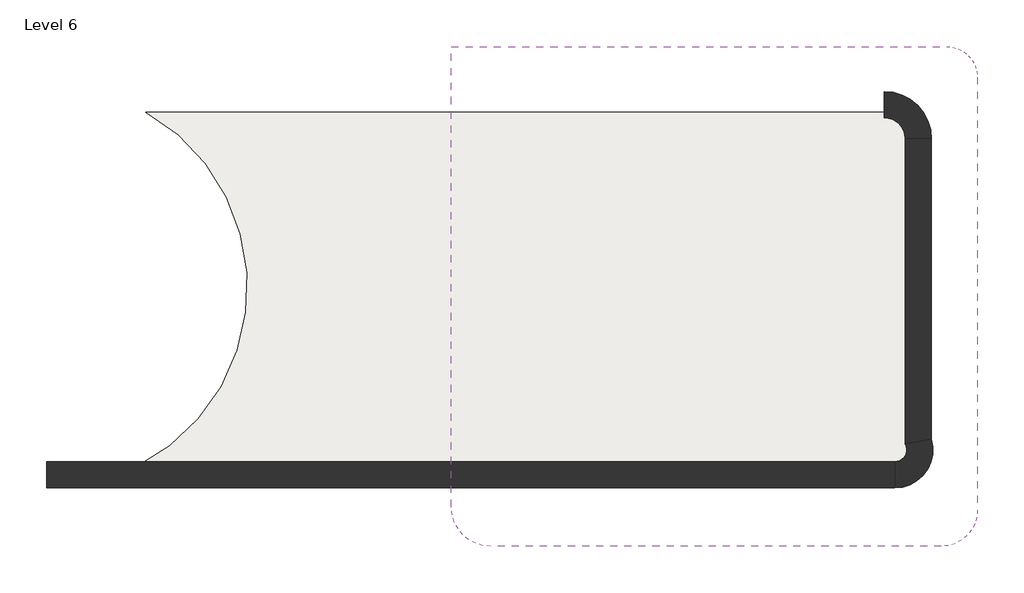
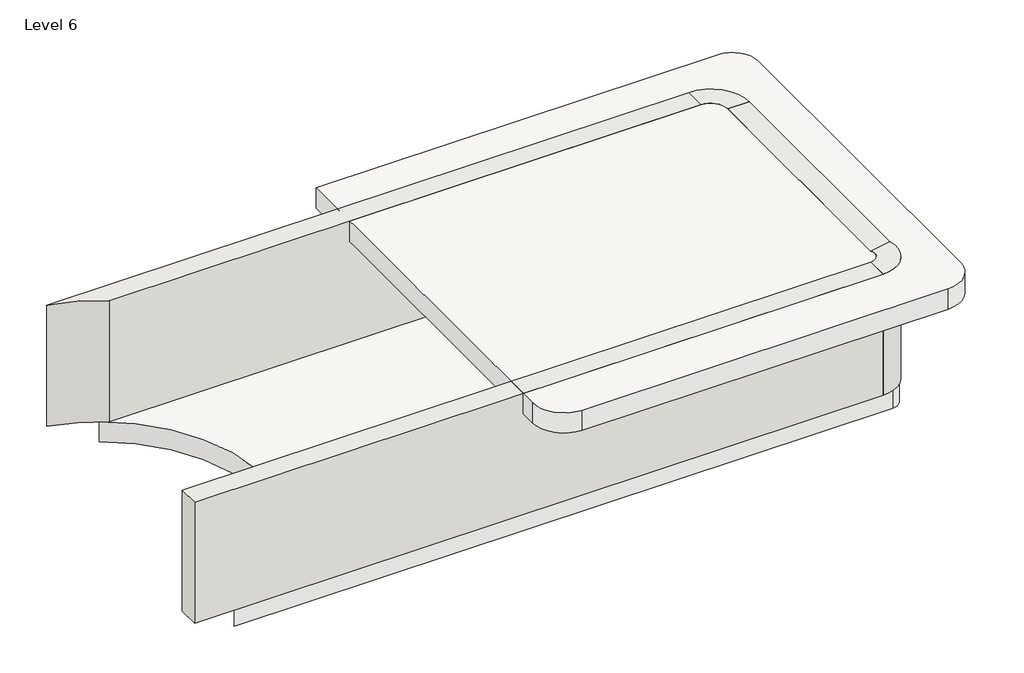
# One storey: 5 walls, 2 slabs.
"""IFC4 building model written with IfcOpenShell, lengths in millimetres."""

from ifc_helpers import new_model, si_unit, point, frame, frame_2d, origin, place, context, project, spatial, polyline, circle_curve, trimmed, segment, composite_curve, outline, extrude, element, save

model = new_model("IFC4")

# Units and contexts
model_context = context("Model", 3, world=origin())
ifc_project = project(units=[si_unit("LENGTHUNIT", "METRE", prefix="MILLI")], contexts=[model_context])

# Site, building, storey
site = spatial("IfcSite", under=ifc_project)
building = spatial("IfcBuilding", under=site)
storey = spatial("IfcBuildingStorey", under=building, Name="Level 6", Elevation=15240.0)

# Slabs
placement = place(None, origin())
element("IfcSlab", 1, ObjectType="Generic - 12\"", at=placement, inside=storey, context=model_context, shape_type="SweptSolid", body=[
    extrude(outline(composite_curve([segment(polyline([(4352.7755462, 9786.507593), (-5048.3861367, 9786.507593)]), True, "CONTINUOUS"), segment(trimmed(circle_curve(frame_2d((-5663.9343196, 12035.4520418)), 2331.662647), [point((-5048.3861367, 9786.507593))], [point((-4509.1659796, 14061.0780636))], True, "CARTESIAN"), True, "CONTINUOUS"), segment(polyline([(-4509.1659796, 14061.0780636), (4330.0340204, 14061.0780636)]), True, "CONTINUOUS"), segment(trimmed(circle_curve(frame_2d((4363.3582159, 13907.657593)), 156.997907), [point((4330.0340204, 14061.0780636))], [point((4520.3561229, 13907.657593))], False, "CARTESIAN"), True, "CONTINUOUS"), segment(polyline([(4520.3561229, 13907.657593), (4520.3561229, 9954.0881697)]), True, "CONTINUOUS"), segment(trimmed(circle_curve(frame_2d((4352.7755462, 9954.0881697)), 167.5805767), [point((4520.3561229, 9954.0881697))], [point((4352.7755462, 9786.507593))], False, "CARTESIAN"), True, "CONTINUOUS")], self_intersect=False)), frame((0.0, 0.0, 14782.8), z_axis=(0.0, 0.0, 1.0), x_axis=(1.0, 0.0, 0.0)), (0.0, 0.0, 1.0), 304.8),
])
element("IfcSlab", 2, ObjectType="Generic - 12\"", at=placement, inside=storey, context=model_context, shape_type="SweptSolid", body=[
    extrude(outline(composite_curve([segment(trimmed(circle_curve(frame_2d((4770.6315344, 14464.0053975)), 355.8514084), [point((4770.6315344, 14819.8568058))], [point((5126.4829427, 14464.0053975))], False, "CARTESIAN"), True, "CONTINUOUS"), segment(polyline([(5126.4829427, 14464.0053975), (5126.4829427, 9448.7477683)]), True, "CONTINUOUS"), segment(trimmed(circle_curve(frame_2d((4706.3919803, 9448.7477683)), 420.0909624), [point((5126.4829427, 9448.7477683))], [point((4706.3919803, 9028.6568058))], False, "CARTESIAN"), True, "CONTINUOUS"), segment(polyline([(4706.3919803, 9028.6568058), (-516.4662702, 9028.6568058)]), True, "CONTINUOUS"), segment(trimmed(circle_curve(frame_2d((-516.4662702, 9481.707593)), 453.0507871), [point((-516.4662702, 9028.6568058))], [point((-969.5170573, 9481.707593))], False, "CARTESIAN"), True, "CONTINUOUS"), segment(polyline([(-969.5170573, 9481.707593), (-969.5170573, 14819.8568058), (4770.6315344, 14819.8568058)]), True, "CONTINUOUS")], self_intersect=False)), frame((0.0, 0.0, 16611.6), z_axis=(0.0, 0.0, 1.0), x_axis=(1.0, 0.0, 0.0)), (0.0, 0.0, 1.0), 304.8),
])

# Walls
element("IfcWall", 3, ObjectType="Generic - 12\" white", at=placement, inside=storey, context=model_context, shape_type="SweptSolid", body=[
    extrude(outline(polyline([(4168.535193, 9704.4209117), (-5661.264807, 9704.4209117), (-5661.264807, 10009.2209117), (4168.535193, 10009.2209117), (4168.535193, 9704.4209117)])), frame((0.0, 0.0, 15087.6), z_axis=(0.0, 0.0, 1.0), x_axis=(1.0, 0.0, 0.0)), (0.0, 0.0, 1.0), 1828.8),
])
element("IfcWall", 4, ObjectType="Generic - 12\" white", at=placement, inside=storey, context=model_context, shape_type="SweptSolid", body=[
    extrude(outline(composite_curve([segment(polyline([(4288.804449, 10214.1868139), (4593.604449, 10270.2090301)]), True, "CONTINUOUS"), segment(trimmed(circle_curve(frame_2d((4168.535193, 10146.9894732)), 442.5685615), [point((4593.604449, 10270.2090301))], [point((4168.535193, 9704.4209117))], False, "CARTESIAN"), True, "CONTINUOUS"), segment(polyline([(4168.535193, 9704.4209117), (4168.535193, 10009.2209117)]), True, "CONTINUOUS"), segment(trimmed(circle_curve(frame_2d((4168.535193, 10146.9894732)), 137.7685615), [point((4168.535193, 10009.2209117))], [point((4288.804449, 10214.1868139))], True, "CARTESIAN"), True, "CONTINUOUS")], self_intersect=False)), frame((0.0, 0.0, 15087.6), z_axis=(0.0, 0.0, 1.0), x_axis=(1.0, 0.0, 0.0)), (0.0, 0.0, 1.0), 1828.8),
])
element("IfcWall", 5, ObjectType="Generic - 12\" white", at=placement, inside=storey, context=model_context, shape_type="SweptSolid", body=[
    extrude(outline(polyline([(4593.604449, 13751.4329662), (4593.604449, 10270.2090301), (4288.804449, 10214.1868139), (4288.804449, 13751.4329662), (4593.604449, 13751.4329662)])), frame((0.0, 0.0, 15087.6), z_axis=(0.0, 0.0, 1.0), x_axis=(1.0, 0.0, 0.0)), (0.0, 0.0, 1.0), 1828.8),
])
element("IfcWall", 6, ObjectType="Generic - 12\" white", at=placement, inside=storey, context=model_context, shape_type="SweptSolid", body=[
    extrude(outline(composite_curve([segment(polyline([(4046.1320177, 13994.1053975), (4046.1320177, 14298.9053975)]), True, "CONTINUOUS"), segment(trimmed(circle_curve(frame_2d((4046.1320177, 13751.4329662)), 547.4724313), [point((4046.1320177, 14298.9053975))], [point((4593.604449, 13751.4329662))], False, "CARTESIAN"), True, "CONTINUOUS"), segment(polyline([(4593.604449, 13751.4329662), (4288.804449, 13751.4329662)]), True, "CONTINUOUS"), segment(trimmed(circle_curve(frame_2d((4046.1320177, 13751.4329662)), 242.6724313), [point((4288.804449, 13751.4329662))], [point((4046.1320177, 13994.1053975))], True, "CARTESIAN"), True, "CONTINUOUS")], self_intersect=False)), frame((0.0, 0.0, 15087.6), z_axis=(0.0, 0.0, 1.0), x_axis=(1.0, 0.0, 0.0)), (0.0, 0.0, 1.0), 1828.8),
])
element("IfcWall", 7, ObjectType="Generic - 12\" white", at=placement, inside=storey, context=model_context, shape_type="SweptSolid", body=[
    extrude(outline(composite_curve([segment(polyline([(-5121.1261536, 14298.9053975), (4046.1320177, 14298.9053975), (4046.1320177, 13994.1053975), (-4404.3277377, 13994.1053975)]), True, "CONTINUOUS"), segment(trimmed(circle_curve(frame_2d((-5661.264807, 12033.4131546)), 2328.9922429), [point((-4404.3277377, 13994.1053975))], [point((-5121.1261536, 14298.9053975))], True, "CARTESIAN"), True, "CONTINUOUS")], self_intersect=False)), frame((0.0, 0.0, 15087.6), z_axis=(0.0, 0.0, 1.0), x_axis=(1.0, 0.0, 0.0)), (0.0, 0.0, 1.0), 1828.8),
])

save(model, "model.ifc")

# Revit data of these elements
# Type "Generic - 12\""
#   Assembly Code = "B1010"
#   Function = 0
#   Layers, outside or top first: 1' - 0" "Door - Frame" (function 1)
# Type "Generic - 12\" white"
#   Assembly Code = "B2010"
#   Layers, outside or top first: 1' - 0" "Door - Frame" (function 1)
# Element 1 (IfcSlab, "Generic - 12\"")
#   Height Offset From Level = -0' - 6"
#   Phase Created = New Construction
#   Materials on its faces: "Door - Frame"
# Element 2 (IfcSlab, "Generic - 12\"")
#   Height Offset From Level = 5' - 6"
#   Phase Created = New Construction
#   Materials on its faces: "Door - Frame"
# Elements 3, 5, 7 (IfcWall, "Generic - 12\" white")
#   built-in parameter 1001111 = -0' - 6"
#   Top Offset = 0' - 0"
#   Base Offset = -0' - 6"
#   Unconnected Height = 6' - 0"
#   wall height = 6' - 0"
#   Phase Created = New Construction
#   Base Constraint = Level 6
#   Materials on its faces: "Door - Frame"
# Elements 4, 6 (IfcWall, "Generic - 12\" white")
#   built-in parameter 1001111 = -0' - 6"
#   Top Offset = 0' - 0"
#   Base Offset = -0' - 6"
#   Unconnected Height = 6' - 0"
#   wall height = 6' - 0"
#   Phase Created = New Construction
#   Materials on its faces: "Door - Frame"
# Materials
#   "Door - Frame": colour RGB 118 70 51, transparency 0, Cost = 0
